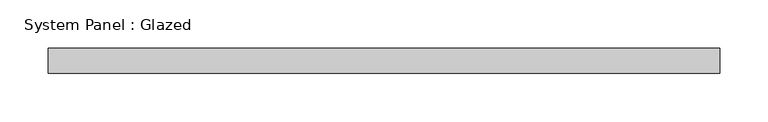
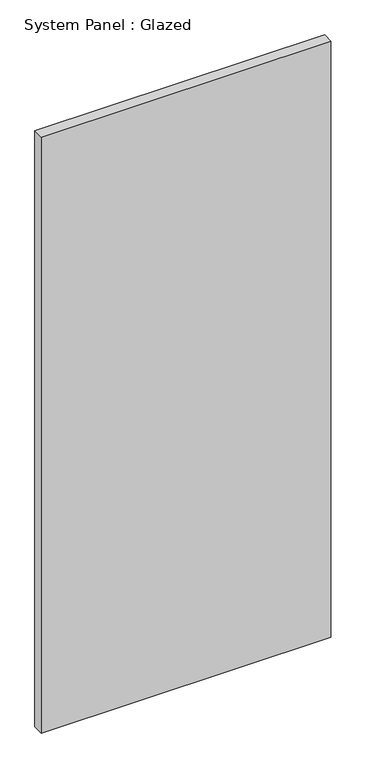
"""IFC4 building model written with IfcOpenShell, lengths in millimetres: plate geometry, System Panel : Glazed."""

from ifc_helpers import new_model, si_unit, origin, origin_with_axes, place, context, project, spatial, polyline, outline, extrude, source, transform, mapped, element, save


def system_panel_glazed_bca51d21(model_context):
    return source(origin(), model_context, "Body", "SweptSolid", [
        extrude(outline(polyline([(346.075, 19.05), (-346.075, 19.05), (-346.075, 44.45), (346.075, 44.45), (346.075, 19.05)])), origin_with_axes(), (0.0, 0.0, 1.0), 1504.45108),
    ])


if __name__ == "__main__":
    model = new_model("IFC4")
    model_context = context("Model", 3, world=origin())
    ifc_project = project(units=[si_unit("LENGTHUNIT", "METRE", prefix="MILLI")], contexts=[model_context])
    site = spatial("IfcSite", under=ifc_project)
    building = spatial("IfcBuilding", under=site)
    placement = place(None, origin())
    system_panel_glazed_shape = system_panel_glazed_bca51d21(model_context)
    element("IfcPlate", 1, ObjectType="System Panel : Glazed", at=placement, inside=building, context=model_context, shape_type="MappedRepresentation", body=[
        mapped(system_panel_glazed_shape, transform((0.0, 0.0, 0.0), x_axis=(1.0, 0.0, 0.0), y_axis=(0.0, 1.0, 0.0), z_axis=(0.0, 0.0, 1.0))),
    ])
    save(model, "model.ifc")

# Revit data of these elements
# Type "System Panel : Glazed"
#   Construction Type Id = "GSP4R"
#   Analytic Construction = "1/8 in Pilkington single glazing"
#   Visual Light Transmittance = 0.9
#   Solar Heat Gain Coefficient = 0.86
#   Heat Transfer Coefficient (U) = 1.18115 BTU/(h·ft²·°F)
#   Define Thermal Properties by = 1
# Element 1 (IfcPlate, "System Panel : Glazed")
#   Materials on its faces: "Glass"
# Materials
#   "Glass": class "Glass", colour RGB 0 128 192, transparency 0.75, Description = "Soda Lime Glass", Cost = 0
